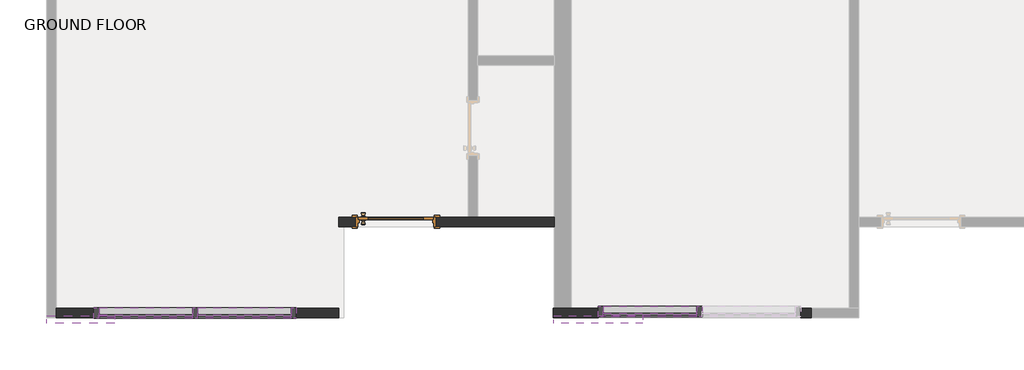
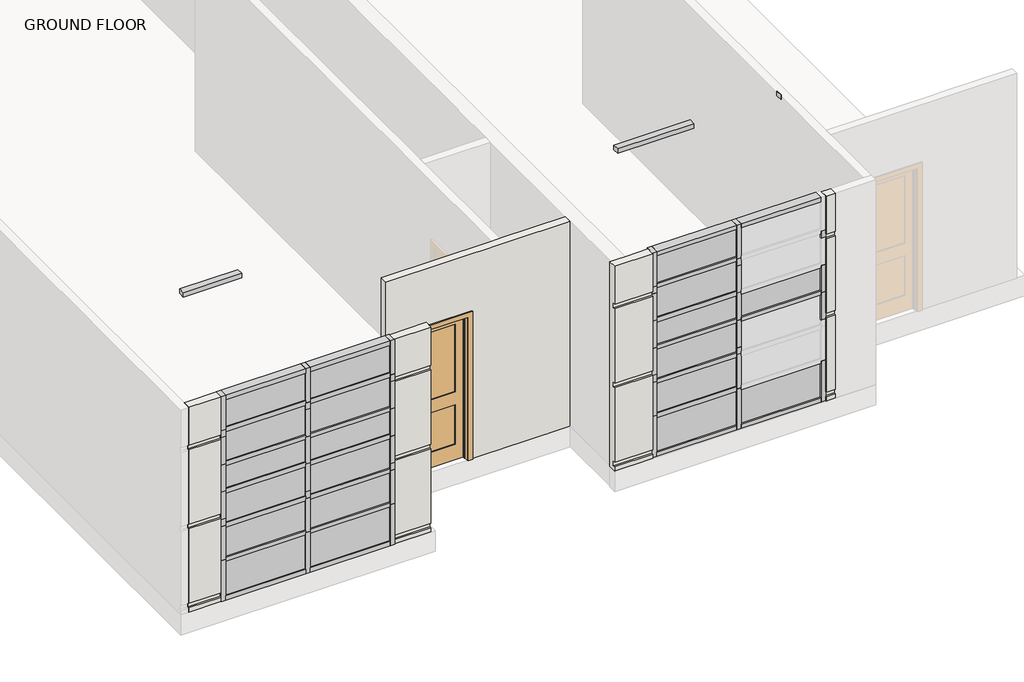
# One storey, part 1 of 4: 68 members, 20 plates, 3 walls, 2 proxies, 1 door.
"""IFC4 building model written with IfcOpenShell, lengths in millimetres."""

from ifc_helpers import new_model, si_unit, frame, origin, place, context, project, spatial, polyline, outline, extrude, faceted_brep, transform, mapped, element, save
from components import door_d4071c8b, member_e6b9f524, member_90c805a2, member_866a01fa, member_7cfea1b5, member_6e77e263, member_47bfaf8a, member_cfc5edb3, member_90750a43, member_7fd687a9, member_fb13da3b, system_panel_glazed_01dbb714, system_panel_glazed_738ee2ab, system_panel_glazed_162183a4, system_panel_glazed_09ecb9ef, system_panel_glazed_28d744da, system_panel_glazed_d671f7fc

model = new_model("IFC4")

# Units and contexts
model_context = context("Model", 3, world=origin())
ifc_project = project(units=[si_unit("LENGTHUNIT", "METRE", prefix="MILLI")], contexts=[model_context])

# Site, building, storey
site = spatial("IfcSite", under=ifc_project)
building = spatial("IfcBuilding", under=site)
storey = spatial("IfcBuildingStorey", under=building, Name="GROUND FLOOR", Elevation=304.8)

# Proxies
placement = place(None, origin())
element("IfcBuildingElementProxy", 1, Name="Reveal 2", ObjectType="Reveal 2", at=placement, inside=storey, context=model_context, shape_type="SweptSolid", body=[
    extrude(outline(polyline([(-18263.2007021, -5496.2840801), (-18263.2007021, -5404.2090801), (-17444.0507021, -5404.2090801), (-17444.0507021, -5496.2840801), (-18263.2007021, -5496.2840801)])), frame((0.0, 0.0, 5072.38), z_axis=(0.0, 0.0, 1.0), x_axis=(1.0, 0.0, 0.0)), (0.0, 0.0, 1.0), 67.7333333),
])
element("IfcBuildingElementProxy", 2, Name="Reveal 2", ObjectType="Reveal 2", at=placement, inside=storey, context=model_context, shape_type="SweptSolid", body=[
    extrude(outline(polyline([(-9849.450702, -5405.2582515), (-9849.450702, -5497.3332515), (-9856.2720515, -5497.3332515), (-9856.2720515, -5405.2582515), (-9849.450702, -5405.2582515)])), frame((0.0, 0.0, 5072.38), z_axis=(0.0, 0.0, 1.0), x_axis=(1.0, 0.0, 0.0)), (0.0, 0.0, 1.0), 67.7333333),
    extrude(outline(polyline([(-11075.4720515, -5405.2582515), (-11075.4720515, -5497.3332515), (-12149.0934009, -5497.3332515), (-12149.0934009, -5405.2582515), (-11075.4720515, -5405.2582515)])), frame((0.0, 0.0, 5072.38), z_axis=(0.0, 0.0, 1.0), x_axis=(1.0, 0.0, 0.0)), (0.0, 0.0, 1.0), 67.7333333),
])

# Door
door_shape = door_d4071c8b(model_context)
element("IfcDoor", 3, ObjectType="Door-Interior-Single-2_Panel-Wood : 36\" x 84\"", at=placement, inside=storey, context=model_context, shape_type="MappedRepresentation", body=[
    mapped(door_shape, transform((-14053.1507021, -4269.409083, 304.8), x_axis=(1.0, 0.0, 0.0), y_axis=(0.0, 1.0, 0.0), z_axis=(0.0, 0.0, 1.0))),
])

# Members
member_shape = member_e6b9f524(model_context)
element("IfcMember", 4, ObjectType="Rectangular Mullion : 2.5\" x 5\" rectangular", at=placement, inside=storey, context=model_context, shape_type="MappedRepresentation", body=[
    mapped(member_shape, transform((-15316.8007021, -5372.4590801, 3352.8), x_axis=(0.0, 0.0, 1.0), y_axis=(0.0, -1.0, 0.0), z_axis=(1.0, 0.0, 0.0))),
])
element("IfcMember", 5, ObjectType="Rectangular Mullion : 2.5\" x 5\" rectangular", at=placement, inside=storey, context=model_context, shape_type="MappedRepresentation", body=[
    mapped(member_shape, transform((-16504.2507021, -5372.4590801, 3352.8), x_axis=(0.0, 0.0, 1.0), y_axis=(0.0, -1.0, 0.0), z_axis=(1.0, 0.0, 0.0))),
])
element("IfcMember", 6, ObjectType="Rectangular Mullion : 2.5\" x 5\" rectangular", at=placement, inside=storey, context=model_context, shape_type="MappedRepresentation", body=[
    mapped(member_shape, transform((-9240.0344894, -5353.4090801, 3352.8), x_axis=(0.0, 0.0, 1.0), y_axis=(0.0, -1.0, 0.0), z_axis=(1.0, 0.0, 0.0))),
])
element("IfcMember", 7, ObjectType="Rectangular Mullion : 2.5\" x 5\" rectangular", at=placement, inside=storey, context=model_context, shape_type="MappedRepresentation", body=[
    mapped(member_shape, transform((-10427.4844894, -5353.4090801, 3352.8), x_axis=(0.0, 0.0, 1.0), y_axis=(0.0, -1.0, 0.0), z_axis=(1.0, 0.0, 0.0))),
])
element("IfcMember", 8, ObjectType="Rectangular Mullion : 2.5\" x 5\" rectangular", at=placement, inside=storey, context=model_context, shape_type="MappedRepresentation", body=[
    mapped(member_shape, transform((-17628.2007021, -5372.4590801, 304.8), x_axis=(0.0, 0.0, -1.0), y_axis=(0.0, -1.0, 0.0), z_axis=(-1.0, 0.0, 0.0))),
])
element("IfcMember", 9, ObjectType="Rectangular Mullion : 2.5\" x 5\" rectangular", at=placement, inside=storey, context=model_context, shape_type="MappedRepresentation", body=[
    mapped(member_shape, transform((-16440.7507021, -5372.4590801, 304.8), x_axis=(0.0, 0.0, -1.0), y_axis=(0.0, -1.0, 0.0), z_axis=(-1.0, 0.0, 0.0))),
])
element("IfcMember", 10, ObjectType="Rectangular Mullion : 2.5\" x 5\" rectangular", at=placement, inside=storey, context=model_context, shape_type="MappedRepresentation", body=[
    mapped(member_shape, transform((-11551.4344894, -5353.4090801, 304.8), x_axis=(0.0, 0.0, -1.0), y_axis=(0.0, -1.0, 0.0), z_axis=(-1.0, 0.0, 0.0))),
])
element("IfcMember", 11, ObjectType="Rectangular Mullion : 2.5\" x 5\" rectangular", at=placement, inside=storey, context=model_context, shape_type="MappedRepresentation", body=[
    mapped(member_shape, transform((-10363.9844894, -5353.4090801, 304.8), x_axis=(0.0, 0.0, -1.0), y_axis=(0.0, -1.0, 0.0), z_axis=(-1.0, 0.0, 0.0))),
])
member_2_shape = member_90c805a2(model_context)
element("IfcMember", 12, ObjectType="Rectangular Mullion : 2.5\" x 5\" rectangular", at=placement, inside=storey, context=model_context, shape_type="MappedRepresentation", body=[
    mapped(member_2_shape, transform((-16472.5007021, -5372.4590801, 1524.0), x_axis=(1.0, 0.0, 0.0), y_axis=(0.0, -1.0, 0.0), z_axis=(0.0, 0.0, -1.0))),
])
element("IfcMember", 13, ObjectType="Rectangular Mullion : 2.5\" x 5\" rectangular", at=placement, inside=storey, context=model_context, shape_type="MappedRepresentation", body=[
    mapped(member_2_shape, transform((-10395.7344894, -5353.4090801, 1524.0), x_axis=(1.0, 0.0, 0.0), y_axis=(0.0, -1.0, 0.0), z_axis=(0.0, 0.0, -1.0))),
])
member_3_shape = member_866a01fa(model_context)
element("IfcMember", 14, ObjectType="Rectangular Mullion : 2.5\" x 5\" rectangular", at=placement, inside=storey, context=model_context, shape_type="MappedRepresentation", body=[
    mapped(member_3_shape, transform((-16504.2507021, -5372.4590801, 1930.4), x_axis=(0.0, 0.0, 1.0), y_axis=(0.0, -1.0, 0.0), z_axis=(1.0, 0.0, 0.0))),
])
element("IfcMember", 15, ObjectType="Rectangular Mullion : 2.5\" x 5\" rectangular", at=placement, inside=storey, context=model_context, shape_type="MappedRepresentation", body=[
    mapped(member_3_shape, transform((-15316.8007021, -5372.4590801, 1930.4), x_axis=(0.0, 0.0, 1.0), y_axis=(0.0, -1.0, 0.0), z_axis=(1.0, 0.0, 0.0))),
])
element("IfcMember", 16, ObjectType="Rectangular Mullion : 2.5\" x 5\" rectangular", at=placement, inside=storey, context=model_context, shape_type="MappedRepresentation", body=[
    mapped(member_3_shape, transform((-16504.2507021, -5372.4590801, 2336.8), x_axis=(0.0, 0.0, 1.0), y_axis=(0.0, -1.0, 0.0), z_axis=(1.0, 0.0, 0.0))),
])
element("IfcMember", 17, ObjectType="Rectangular Mullion : 2.5\" x 5\" rectangular", at=placement, inside=storey, context=model_context, shape_type="MappedRepresentation", body=[
    mapped(member_3_shape, transform((-15316.8007021, -5372.4590801, 2336.8), x_axis=(0.0, 0.0, 1.0), y_axis=(0.0, -1.0, 0.0), z_axis=(1.0, 0.0, 0.0))),
])
element("IfcMember", 18, ObjectType="Rectangular Mullion : 2.5\" x 5\" rectangular", at=placement, inside=storey, context=model_context, shape_type="MappedRepresentation", body=[
    mapped(member_3_shape, transform((-16504.2507021, -5372.4590801, 914.4), x_axis=(0.0, 0.0, 1.0), y_axis=(0.0, -1.0, 0.0), z_axis=(1.0, 0.0, 0.0))),
])
element("IfcMember", 19, ObjectType="Rectangular Mullion : 2.5\" x 5\" rectangular", at=placement, inside=storey, context=model_context, shape_type="MappedRepresentation", body=[
    mapped(member_3_shape, transform((-15316.8007021, -5372.4590801, 914.4), x_axis=(0.0, 0.0, 1.0), y_axis=(0.0, -1.0, 0.0), z_axis=(1.0, 0.0, 0.0))),
])
element("IfcMember", 20, ObjectType="Rectangular Mullion : 2.5\" x 5\" rectangular", at=placement, inside=storey, context=model_context, shape_type="MappedRepresentation", body=[
    mapped(member_3_shape, transform((-16504.2507021, -5372.4590801, 2844.8), x_axis=(0.0, 0.0, 1.0), y_axis=(0.0, -1.0, 0.0), z_axis=(1.0, 0.0, 0.0))),
])
element("IfcMember", 21, ObjectType="Rectangular Mullion : 2.5\" x 5\" rectangular", at=placement, inside=storey, context=model_context, shape_type="MappedRepresentation", body=[
    mapped(member_3_shape, transform((-15316.8007021, -5372.4590801, 2844.8), x_axis=(0.0, 0.0, 1.0), y_axis=(0.0, -1.0, 0.0), z_axis=(1.0, 0.0, 0.0))),
])
element("IfcMember", 22, ObjectType="Rectangular Mullion : 2.5\" x 5\" rectangular", at=placement, inside=storey, context=model_context, shape_type="MappedRepresentation", body=[
    mapped(member_3_shape, transform((-16504.2507021, -5372.4590801, 1422.4), x_axis=(0.0, 0.0, 1.0), y_axis=(0.0, -1.0, 0.0), z_axis=(1.0, 0.0, 0.0))),
])
element("IfcMember", 23, ObjectType="Rectangular Mullion : 2.5\" x 5\" rectangular", at=placement, inside=storey, context=model_context, shape_type="MappedRepresentation", body=[
    mapped(member_3_shape, transform((-15316.8007021, -5372.4590801, 1422.4), x_axis=(0.0, 0.0, 1.0), y_axis=(0.0, -1.0, 0.0), z_axis=(1.0, 0.0, 0.0))),
])
element("IfcMember", 24, ObjectType="Rectangular Mullion : 2.5\" x 5\" rectangular", at=placement, inside=storey, context=model_context, shape_type="MappedRepresentation", body=[
    mapped(member_3_shape, transform((-10427.4844894, -5353.4090801, 1930.4), x_axis=(0.0, 0.0, 1.0), y_axis=(0.0, -1.0, 0.0), z_axis=(1.0, 0.0, 0.0))),
])
element("IfcMember", 25, ObjectType="Rectangular Mullion : 2.5\" x 5\" rectangular", at=placement, inside=storey, context=model_context, shape_type="MappedRepresentation", body=[
    mapped(member_3_shape, transform((-9240.0344894, -5353.4090801, 1930.4), x_axis=(0.0, 0.0, 1.0), y_axis=(0.0, -1.0, 0.0), z_axis=(1.0, 0.0, 0.0))),
])
element("IfcMember", 26, ObjectType="Rectangular Mullion : 2.5\" x 5\" rectangular", at=placement, inside=storey, context=model_context, shape_type="MappedRepresentation", body=[
    mapped(member_3_shape, transform((-10427.4844894, -5353.4090801, 2336.8), x_axis=(0.0, 0.0, 1.0), y_axis=(0.0, -1.0, 0.0), z_axis=(1.0, 0.0, 0.0))),
])
element("IfcMember", 27, ObjectType="Rectangular Mullion : 2.5\" x 5\" rectangular", at=placement, inside=storey, context=model_context, shape_type="MappedRepresentation", body=[
    mapped(member_3_shape, transform((-10427.4844894, -5353.4090801, 914.4), x_axis=(0.0, 0.0, 1.0), y_axis=(0.0, -1.0, 0.0), z_axis=(1.0, 0.0, 0.0))),
])
element("IfcMember", 28, ObjectType="Rectangular Mullion : 2.5\" x 5\" rectangular", at=placement, inside=storey, context=model_context, shape_type="MappedRepresentation", body=[
    mapped(member_3_shape, transform((-10427.4844894, -5353.4090801, 2844.8), x_axis=(0.0, 0.0, 1.0), y_axis=(0.0, -1.0, 0.0), z_axis=(1.0, 0.0, 0.0))),
])
element("IfcMember", 29, ObjectType="Rectangular Mullion : 2.5\" x 5\" rectangular", at=placement, inside=storey, context=model_context, shape_type="MappedRepresentation", body=[
    mapped(member_3_shape, transform((-10427.4844894, -5353.4090801, 1422.4), x_axis=(0.0, 0.0, 1.0), y_axis=(0.0, -1.0, 0.0), z_axis=(1.0, 0.0, 0.0))),
])
member_4_shape = member_7cfea1b5(model_context)
element("IfcMember", 30, ObjectType="Rectangular Mullion : 2.5\" x 5\" rectangular", at=placement, inside=storey, context=model_context, shape_type="MappedRepresentation", body=[
    mapped(member_4_shape, transform((-15253.3007021, -5372.4590801, 1524.0), x_axis=(1.0, 0.0, 0.0), y_axis=(0.0, -1.0, 0.0), z_axis=(0.0, 0.0, -1.0))),
])
element("IfcMember", 31, ObjectType="Rectangular Mullion : 2.5\" x 5\" rectangular", at=placement, inside=storey, context=model_context, shape_type="MappedRepresentation", body=[
    mapped(member_4_shape, transform((-9176.5344894, -5353.4090801, 1524.0), x_axis=(1.0, 0.0, 0.0), y_axis=(0.0, -1.0, 0.0), z_axis=(0.0, 0.0, -1.0))),
])
element("IfcMember", 32, ObjectType="Rectangular Mullion : 2.5\" x 5\" rectangular", at=placement, inside=storey, context=model_context, shape_type="MappedRepresentation", body=[
    mapped(member_4_shape, transform((-17691.7007021, -5372.4590801, 1930.4), x_axis=(-1.0, 0.0, 0.0), y_axis=(0.0, -1.0, 0.0), z_axis=(0.0, 0.0, 1.0))),
])
element("IfcMember", 33, ObjectType="Rectangular Mullion : 2.5\" x 5\" rectangular", at=placement, inside=storey, context=model_context, shape_type="MappedRepresentation", body=[
    mapped(member_4_shape, transform((-11614.9344894, -5353.4090801, 1930.4), x_axis=(-1.0, 0.0, 0.0), y_axis=(0.0, -1.0, 0.0), z_axis=(0.0, 0.0, 1.0))),
])
element("IfcMember", 34, ObjectType="Rectangular Mullion : 2.5\" x 5\" rectangular", at=placement, inside=storey, context=model_context, shape_type="MappedRepresentation", body=[
    mapped(member_2_shape, transform((-16472.5007021, -5372.4590801, 1930.4), x_axis=(1.0, 0.0, 0.0), y_axis=(0.0, -1.0, 0.0), z_axis=(0.0, 0.0, -1.0))),
])
element("IfcMember", 35, ObjectType="Rectangular Mullion : 2.5\" x 5\" rectangular", at=placement, inside=storey, context=model_context, shape_type="MappedRepresentation", body=[
    mapped(member_2_shape, transform((-10395.7344894, -5353.4090801, 1930.4), x_axis=(1.0, 0.0, 0.0), y_axis=(0.0, -1.0, 0.0), z_axis=(0.0, 0.0, -1.0))),
])
element("IfcMember", 36, ObjectType="Rectangular Mullion : 2.5\" x 5\" rectangular", at=placement, inside=storey, context=model_context, shape_type="MappedRepresentation", body=[
    mapped(member_2_shape, transform((-16472.5007021, -5372.4590801, 2336.8), x_axis=(1.0, 0.0, 0.0), y_axis=(0.0, -1.0, 0.0), z_axis=(0.0, 0.0, -1.0))),
])
element("IfcMember", 37, ObjectType="Rectangular Mullion : 2.5\" x 5\" rectangular", at=placement, inside=storey, context=model_context, shape_type="MappedRepresentation", body=[
    mapped(member_2_shape, transform((-10395.7344894, -5353.4090801, 2336.8), x_axis=(1.0, 0.0, 0.0), y_axis=(0.0, -1.0, 0.0), z_axis=(0.0, 0.0, -1.0))),
])
element("IfcMember", 38, ObjectType="Rectangular Mullion : 2.5\" x 5\" rectangular", at=placement, inside=storey, context=model_context, shape_type="MappedRepresentation", body=[
    mapped(member_4_shape, transform((-17691.7007021, -5372.4590801, 2743.2), x_axis=(-1.0, 0.0, 0.0), y_axis=(0.0, -1.0, 0.0), z_axis=(0.0, 0.0, 1.0))),
])
element("IfcMember", 39, ObjectType="Rectangular Mullion : 2.5\" x 5\" rectangular", at=placement, inside=storey, context=model_context, shape_type="MappedRepresentation", body=[
    mapped(member_4_shape, transform((-11614.9344894, -5353.4090801, 2743.2), x_axis=(-1.0, 0.0, 0.0), y_axis=(0.0, -1.0, 0.0), z_axis=(0.0, 0.0, 1.0))),
])
element("IfcMember", 40, ObjectType="Rectangular Mullion : 2.5\" x 5\" rectangular", at=placement, inside=storey, context=model_context, shape_type="MappedRepresentation", body=[
    mapped(member_4_shape, transform((-15253.3007021, -5372.4590801, 1930.4), x_axis=(1.0, 0.0, 0.0), y_axis=(0.0, -1.0, 0.0), z_axis=(0.0, 0.0, -1.0))),
])
element("IfcMember", 41, ObjectType="Rectangular Mullion : 2.5\" x 5\" rectangular", at=placement, inside=storey, context=model_context, shape_type="MappedRepresentation", body=[
    mapped(member_4_shape, transform((-9176.5344894, -5353.4090801, 1930.4), x_axis=(1.0, 0.0, 0.0), y_axis=(0.0, -1.0, 0.0), z_axis=(0.0, 0.0, -1.0))),
])
element("IfcMember", 42, ObjectType="Rectangular Mullion : 2.5\" x 5\" rectangular", at=placement, inside=storey, context=model_context, shape_type="MappedRepresentation", body=[
    mapped(member_4_shape, transform((-15253.3007021, -5372.4590801, 2336.8), x_axis=(1.0, 0.0, 0.0), y_axis=(0.0, -1.0, 0.0), z_axis=(0.0, 0.0, -1.0))),
])
element("IfcMember", 43, ObjectType="Rectangular Mullion : 2.5\" x 5\" rectangular", at=placement, inside=storey, context=model_context, shape_type="MappedRepresentation", body=[
    mapped(member_4_shape, transform((-17691.7007021, -5372.4590801, 2336.8), x_axis=(-1.0, 0.0, 0.0), y_axis=(0.0, -1.0, 0.0), z_axis=(0.0, 0.0, 1.0))),
])
element("IfcMember", 44, ObjectType="Rectangular Mullion : 2.5\" x 5\" rectangular", at=placement, inside=storey, context=model_context, shape_type="MappedRepresentation", body=[
    mapped(member_4_shape, transform((-11614.9344894, -5353.4090801, 2336.8), x_axis=(-1.0, 0.0, 0.0), y_axis=(0.0, -1.0, 0.0), z_axis=(0.0, 0.0, 1.0))),
])
member_5_shape = member_6e77e263(model_context)
element("IfcMember", 45, ObjectType="Rectangular Mullion : 2.5\" x 5\" rectangular", at=placement, inside=storey, context=model_context, shape_type="MappedRepresentation", body=[
    mapped(member_5_shape, transform((-16472.5007021, -5372.4590801, 304.8), x_axis=(1.0, 0.0, 0.0), y_axis=(0.0, -1.0, 0.0), z_axis=(0.0, 0.0, -1.0))),
])
element("IfcMember", 46, ObjectType="Rectangular Mullion : 2.5\" x 5\" rectangular", at=placement, inside=storey, context=model_context, shape_type="MappedRepresentation", body=[
    mapped(member_5_shape, transform((-10395.7344894, -5353.4090801, 304.8), x_axis=(1.0, 0.0, 0.0), y_axis=(0.0, -1.0, 0.0), z_axis=(0.0, 0.0, -1.0))),
])
member_6_shape = member_47bfaf8a(model_context)
element("IfcMember", 47, ObjectType="Rectangular Mullion : 2.5\" x 5\" rectangular", at=placement, inside=storey, context=model_context, shape_type="MappedRepresentation", body=[
    mapped(member_6_shape, transform((-15253.3007021, -5372.4590801, 304.8), x_axis=(1.0, 0.0, 0.0), y_axis=(0.0, -1.0, 0.0), z_axis=(0.0, 0.0, -1.0))),
])
element("IfcMember", 48, ObjectType="Rectangular Mullion : 2.5\" x 5\" rectangular", at=placement, inside=storey, context=model_context, shape_type="MappedRepresentation", body=[
    mapped(member_6_shape, transform((-9176.5344894, -5353.4090801, 304.8), x_axis=(1.0, 0.0, 0.0), y_axis=(0.0, -1.0, 0.0), z_axis=(0.0, 0.0, -1.0))),
])
element("IfcMember", 49, ObjectType="Rectangular Mullion : 2.5\" x 5\" rectangular", at=placement, inside=storey, context=model_context, shape_type="MappedRepresentation", body=[
    mapped(member_6_shape, transform((-17691.7007021, -5372.4590801, 914.4), x_axis=(-1.0, 0.0, 0.0), y_axis=(0.0, -1.0, 0.0), z_axis=(0.0, 0.0, 1.0))),
])
element("IfcMember", 50, ObjectType="Rectangular Mullion : 2.5\" x 5\" rectangular", at=placement, inside=storey, context=model_context, shape_type="MappedRepresentation", body=[
    mapped(member_6_shape, transform((-11614.9344894, -5353.4090801, 914.4), x_axis=(-1.0, 0.0, 0.0), y_axis=(0.0, -1.0, 0.0), z_axis=(0.0, 0.0, 1.0))),
])
member_7_shape = member_cfc5edb3(model_context)
element("IfcMember", 51, ObjectType="Rectangular Mullion : 2.5\" x 5\" rectangular", at=placement, inside=storey, context=model_context, shape_type="MappedRepresentation", body=[
    mapped(member_7_shape, transform((-16472.5007021, -5372.4590801, 2743.2), x_axis=(1.0, 0.0, 0.0), y_axis=(0.0, -1.0, 0.0), z_axis=(0.0, 0.0, -1.0))),
])
element("IfcMember", 52, ObjectType="Rectangular Mullion : 2.5\" x 5\" rectangular", at=placement, inside=storey, context=model_context, shape_type="MappedRepresentation", body=[
    mapped(member_7_shape, transform((-10395.7344894, -5353.4090801, 2743.2), x_axis=(1.0, 0.0, 0.0), y_axis=(0.0, -1.0, 0.0), z_axis=(0.0, 0.0, -1.0))),
])
member_8_shape = member_90750a43(model_context)
element("IfcMember", 53, ObjectType="Rectangular Mullion : 2.5\" x 5\" rectangular", at=placement, inside=storey, context=model_context, shape_type="MappedRepresentation", body=[
    mapped(member_8_shape, transform((-16472.5007021, -5372.4590801, 2844.8), x_axis=(1.0, 0.0, 0.0), y_axis=(0.0, -1.0, 0.0), z_axis=(0.0, 0.0, -1.0))),
])
element("IfcMember", 54, ObjectType="Rectangular Mullion : 2.5\" x 5\" rectangular", at=placement, inside=storey, context=model_context, shape_type="MappedRepresentation", body=[
    mapped(member_8_shape, transform((-10395.7344894, -5353.4090801, 2844.8), x_axis=(1.0, 0.0, 0.0), y_axis=(0.0, -1.0, 0.0), z_axis=(0.0, 0.0, -1.0))),
])
member_9_shape = member_7fd687a9(model_context)
element("IfcMember", 55, ObjectType="Rectangular Mullion : 2.5\" x 5\" rectangular", at=placement, inside=storey, context=model_context, shape_type="MappedRepresentation", body=[
    mapped(member_9_shape, transform((-17691.7007021, -5372.4590801, 3352.8), x_axis=(-1.0, 0.0, 0.0), y_axis=(0.0, -1.0, 0.0), z_axis=(0.0, 0.0, 1.0))),
])
element("IfcMember", 56, ObjectType="Rectangular Mullion : 2.5\" x 5\" rectangular", at=placement, inside=storey, context=model_context, shape_type="MappedRepresentation", body=[
    mapped(member_9_shape, transform((-11614.9344894, -5353.4090801, 3352.8), x_axis=(-1.0, 0.0, 0.0), y_axis=(0.0, -1.0, 0.0), z_axis=(0.0, 0.0, 1.0))),
])
member_10_shape = member_fb13da3b(model_context)
element("IfcMember", 57, ObjectType="Rectangular Mullion : 2.5\" x 5\" rectangular", at=placement, inside=storey, context=model_context, shape_type="MappedRepresentation", body=[
    mapped(member_10_shape, transform((-15253.3007021, -5372.4590801, 2743.2), x_axis=(1.0, 0.0, 0.0), y_axis=(0.0, -1.0, 0.0), z_axis=(0.0, 0.0, -1.0))),
])
element("IfcMember", 58, ObjectType="Rectangular Mullion : 2.5\" x 5\" rectangular", at=placement, inside=storey, context=model_context, shape_type="MappedRepresentation", body=[
    mapped(member_10_shape, transform((-9176.5344894, -5353.4090801, 2743.2), x_axis=(1.0, 0.0, 0.0), y_axis=(0.0, -1.0, 0.0), z_axis=(0.0, 0.0, -1.0))),
])
element("IfcMember", 59, ObjectType="Rectangular Mullion : 2.5\" x 5\" rectangular", at=placement, inside=storey, context=model_context, shape_type="MappedRepresentation", body=[
    mapped(member_9_shape, transform((-15253.3007021, -5372.4590801, 2844.8), x_axis=(1.0, 0.0, 0.0), y_axis=(0.0, -1.0, 0.0), z_axis=(0.0, 0.0, -1.0))),
])
element("IfcMember", 60, ObjectType="Rectangular Mullion : 2.5\" x 5\" rectangular", at=placement, inside=storey, context=model_context, shape_type="MappedRepresentation", body=[
    mapped(member_10_shape, transform((-17691.7007021, -5372.4590801, 2844.8), x_axis=(-1.0, 0.0, 0.0), y_axis=(0.0, -1.0, 0.0), z_axis=(0.0, 0.0, 1.0))),
])
element("IfcMember", 61, ObjectType="Rectangular Mullion : 2.5\" x 5\" rectangular", at=placement, inside=storey, context=model_context, shape_type="MappedRepresentation", body=[
    mapped(member_10_shape, transform((-11614.9344894, -5353.4090801, 2844.8), x_axis=(-1.0, 0.0, 0.0), y_axis=(0.0, -1.0, 0.0), z_axis=(0.0, 0.0, 1.0))),
])
element("IfcMember", 62, ObjectType="Rectangular Mullion : 2.5\" x 5\" rectangular", at=placement, inside=storey, context=model_context, shape_type="MappedRepresentation", body=[
    mapped(member_8_shape, transform((-16472.5007021, -5372.4590801, 914.4), x_axis=(1.0, 0.0, 0.0), y_axis=(0.0, -1.0, 0.0), z_axis=(0.0, 0.0, -1.0))),
])
element("IfcMember", 63, ObjectType="Rectangular Mullion : 2.5\" x 5\" rectangular", at=placement, inside=storey, context=model_context, shape_type="MappedRepresentation", body=[
    mapped(member_8_shape, transform((-10395.7344894, -5353.4090801, 914.4), x_axis=(1.0, 0.0, 0.0), y_axis=(0.0, -1.0, 0.0), z_axis=(0.0, 0.0, -1.0))),
])
element("IfcMember", 64, ObjectType="Rectangular Mullion : 2.5\" x 5\" rectangular", at=placement, inside=storey, context=model_context, shape_type="MappedRepresentation", body=[
    mapped(member_7_shape, transform((-16472.5007021, -5372.4590801, 1422.4), x_axis=(1.0, 0.0, 0.0), y_axis=(0.0, -1.0, 0.0), z_axis=(0.0, 0.0, -1.0))),
])
element("IfcMember", 65, ObjectType="Rectangular Mullion : 2.5\" x 5\" rectangular", at=placement, inside=storey, context=model_context, shape_type="MappedRepresentation", body=[
    mapped(member_7_shape, transform((-10395.7344894, -5353.4090801, 1422.4), x_axis=(1.0, 0.0, 0.0), y_axis=(0.0, -1.0, 0.0), z_axis=(0.0, 0.0, -1.0))),
])
element("IfcMember", 66, ObjectType="Rectangular Mullion : 2.5\" x 5\" rectangular", at=placement, inside=storey, context=model_context, shape_type="MappedRepresentation", body=[
    mapped(member_10_shape, transform((-17691.7007021, -5372.4590801, 1524.0), x_axis=(-1.0, 0.0, 0.0), y_axis=(0.0, -1.0, 0.0), z_axis=(0.0, 0.0, 1.0))),
])
element("IfcMember", 67, ObjectType="Rectangular Mullion : 2.5\" x 5\" rectangular", at=placement, inside=storey, context=model_context, shape_type="MappedRepresentation", body=[
    mapped(member_10_shape, transform((-11614.9344894, -5353.4090801, 1524.0), x_axis=(-1.0, 0.0, 0.0), y_axis=(0.0, -1.0, 0.0), z_axis=(0.0, 0.0, 1.0))),
])
element("IfcMember", 68, ObjectType="Rectangular Mullion : 2.5\" x 5\" rectangular", at=placement, inside=storey, context=model_context, shape_type="MappedRepresentation", body=[
    mapped(member_9_shape, transform((-15253.3007021, -5372.4590801, 914.4), x_axis=(1.0, 0.0, 0.0), y_axis=(0.0, -1.0, 0.0), z_axis=(0.0, 0.0, -1.0))),
])
element("IfcMember", 69, ObjectType="Rectangular Mullion : 2.5\" x 5\" rectangular", at=placement, inside=storey, context=model_context, shape_type="MappedRepresentation", body=[
    mapped(member_10_shape, transform((-15253.3007021, -5372.4590801, 1422.4), x_axis=(1.0, 0.0, 0.0), y_axis=(0.0, -1.0, 0.0), z_axis=(0.0, 0.0, -1.0))),
])
element("IfcMember", 70, ObjectType="Rectangular Mullion : 2.5\" x 5\" rectangular", at=placement, inside=storey, context=model_context, shape_type="MappedRepresentation", body=[
    mapped(member_9_shape, transform((-17691.7007021, -5372.4590801, 1422.4), x_axis=(-1.0, 0.0, 0.0), y_axis=(0.0, -1.0, 0.0), z_axis=(0.0, 0.0, 1.0))),
])
element("IfcMember", 71, ObjectType="Rectangular Mullion : 2.5\" x 5\" rectangular", at=placement, inside=storey, context=model_context, shape_type="MappedRepresentation", body=[
    mapped(member_9_shape, transform((-11614.9344894, -5353.4090801, 1422.4), x_axis=(-1.0, 0.0, 0.0), y_axis=(0.0, -1.0, 0.0), z_axis=(0.0, 0.0, 1.0))),
])

# Plates
system_panel_glazed_shape = system_panel_glazed_01dbb714(model_context)
element("IfcPlate", 72, ObjectType="System Panel : Glazed", at=placement, inside=storey, context=model_context, shape_type="MappedRepresentation", body=[
    mapped(system_panel_glazed_shape, transform((-17066.2257021, -5372.4590801, 1962.15), x_axis=(1.0, 0.0, 0.0), y_axis=(0.0, 1.0, 0.0), z_axis=(0.0, 0.0, 1.0))),
])
element("IfcPlate", 73, ObjectType="System Panel : Glazed", at=placement, inside=storey, context=model_context, shape_type="MappedRepresentation", body=[
    mapped(system_panel_glazed_shape, transform((-15878.7757021, -5372.4590801, 1962.15), x_axis=(1.0, 0.0, 0.0), y_axis=(0.0, 1.0, 0.0), z_axis=(0.0, 0.0, 1.0))),
])
element("IfcPlate", 74, ObjectType="System Panel : Glazed", at=placement, inside=storey, context=model_context, shape_type="MappedRepresentation", body=[
    mapped(system_panel_glazed_shape, transform((-10989.4594894, -5353.4090801, 1962.15), x_axis=(1.0, 0.0, 0.0), y_axis=(0.0, 1.0, 0.0), z_axis=(0.0, 0.0, 1.0))),
])
element("IfcPlate", 75, ObjectType="System Panel : Glazed", at=placement, inside=storey, context=model_context, shape_type="MappedRepresentation", body=[
    mapped(system_panel_glazed_shape, transform((-9802.0094894, -5353.4090801, 1962.15), x_axis=(1.0, 0.0, 0.0), y_axis=(0.0, 1.0, 0.0), z_axis=(0.0, 0.0, 1.0))),
])
system_panel_glazed_2_shape = system_panel_glazed_738ee2ab(model_context)
element("IfcPlate", 76, ObjectType="System Panel : Glazed", at=placement, inside=storey, context=model_context, shape_type="MappedRepresentation", body=[
    mapped(system_panel_glazed_2_shape, transform((-17066.2257021, -5372.4590801, 368.3), x_axis=(1.0, 0.0, 0.0), y_axis=(0.0, 1.0, 0.0), z_axis=(0.0, 0.0, 1.0))),
])
element("IfcPlate", 77, ObjectType="System Panel : Glazed", at=placement, inside=storey, context=model_context, shape_type="MappedRepresentation", body=[
    mapped(system_panel_glazed_2_shape, transform((-15878.7757021, -5372.4590801, 368.3), x_axis=(1.0, 0.0, 0.0), y_axis=(0.0, 1.0, 0.0), z_axis=(0.0, 0.0, 1.0))),
])
element("IfcPlate", 78, ObjectType="System Panel : Glazed", at=placement, inside=storey, context=model_context, shape_type="MappedRepresentation", body=[
    mapped(system_panel_glazed_2_shape, transform((-10989.4594894, -5353.4090801, 368.3), x_axis=(1.0, 0.0, 0.0), y_axis=(0.0, 1.0, 0.0), z_axis=(0.0, 0.0, 1.0))),
])
element("IfcPlate", 79, ObjectType="System Panel : Glazed", at=placement, inside=storey, context=model_context, shape_type="MappedRepresentation", body=[
    mapped(system_panel_glazed_2_shape, transform((-9802.0094894, -5353.4090801, 368.3), x_axis=(1.0, 0.0, 0.0), y_axis=(0.0, 1.0, 0.0), z_axis=(0.0, 0.0, 1.0))),
])
system_panel_glazed_3_shape = system_panel_glazed_162183a4(model_context)
element("IfcPlate", 80, ObjectType="System Panel : Glazed", at=placement, inside=storey, context=model_context, shape_type="MappedRepresentation", body=[
    mapped(system_panel_glazed_3_shape, transform((-17066.2257021, -5372.4590801, 2368.55), x_axis=(1.0, 0.0, 0.0), y_axis=(0.0, 1.0, 0.0), z_axis=(0.0, 0.0, 1.0))),
])
element("IfcPlate", 81, ObjectType="System Panel : Glazed", at=placement, inside=storey, context=model_context, shape_type="MappedRepresentation", body=[
    mapped(system_panel_glazed_3_shape, transform((-15878.7757021, -5372.4590801, 2368.55), x_axis=(1.0, 0.0, 0.0), y_axis=(0.0, 1.0, 0.0), z_axis=(0.0, 0.0, 1.0))),
])
element("IfcPlate", 82, ObjectType="System Panel : Glazed", at=placement, inside=storey, context=model_context, shape_type="MappedRepresentation", body=[
    mapped(system_panel_glazed_3_shape, transform((-10989.4594894, -5353.4090801, 2368.55), x_axis=(1.0, 0.0, 0.0), y_axis=(0.0, 1.0, 0.0), z_axis=(0.0, 0.0, 1.0))),
])
system_panel_glazed_4_shape = system_panel_glazed_09ecb9ef(model_context)
element("IfcPlate", 83, ObjectType="System Panel : Glazed", at=placement, inside=storey, context=model_context, shape_type="MappedRepresentation", body=[
    mapped(system_panel_glazed_4_shape, transform((-17066.2257021, -5372.4590801, 2876.55), x_axis=(1.0, 0.0, 0.0), y_axis=(0.0, 1.0, 0.0), z_axis=(0.0, 0.0, 1.0))),
])
element("IfcPlate", 84, ObjectType="System Panel : Glazed", at=placement, inside=storey, context=model_context, shape_type="MappedRepresentation", body=[
    mapped(system_panel_glazed_4_shape, transform((-15878.7757021, -5372.4590801, 2876.55), x_axis=(1.0, 0.0, 0.0), y_axis=(0.0, 1.0, 0.0), z_axis=(0.0, 0.0, 1.0))),
])
element("IfcPlate", 85, ObjectType="System Panel : Glazed", at=placement, inside=storey, context=model_context, shape_type="MappedRepresentation", body=[
    mapped(system_panel_glazed_4_shape, transform((-10989.4594894, -5353.4090801, 2876.55), x_axis=(1.0, 0.0, 0.0), y_axis=(0.0, 1.0, 0.0), z_axis=(0.0, 0.0, 1.0))),
])
system_panel_glazed_5_shape = system_panel_glazed_28d744da(model_context)
element("IfcPlate", 86, ObjectType="System Panel : Glazed", at=placement, inside=storey, context=model_context, shape_type="MappedRepresentation", body=[
    mapped(system_panel_glazed_5_shape, transform((-17066.2257021, -5372.4590801, 946.15), x_axis=(1.0, 0.0, 0.0), y_axis=(0.0, 1.0, 0.0), z_axis=(0.0, 0.0, 1.0))),
])
element("IfcPlate", 87, ObjectType="System Panel : Glazed", at=placement, inside=storey, context=model_context, shape_type="MappedRepresentation", body=[
    mapped(system_panel_glazed_5_shape, transform((-15878.7757021, -5372.4590801, 946.15), x_axis=(1.0, 0.0, 0.0), y_axis=(0.0, 1.0, 0.0), z_axis=(0.0, 0.0, 1.0))),
])
element("IfcPlate", 88, ObjectType="System Panel : Glazed", at=placement, inside=storey, context=model_context, shape_type="MappedRepresentation", body=[
    mapped(system_panel_glazed_5_shape, transform((-10989.4594894, -5353.4090801, 946.15), x_axis=(1.0, 0.0, 0.0), y_axis=(0.0, 1.0, 0.0), z_axis=(0.0, 0.0, 1.0))),
])
system_panel_glazed_6_shape = system_panel_glazed_d671f7fc(model_context)
element("IfcPlate", 89, ObjectType="System Panel : Glazed", at=placement, inside=storey, context=model_context, shape_type="MappedRepresentation", body=[
    mapped(system_panel_glazed_6_shape, transform((-17066.2257021, -5372.4590801, 1454.15), x_axis=(1.0, 0.0, 0.0), y_axis=(0.0, 1.0, 0.0), z_axis=(0.0, 0.0, 1.0))),
])
element("IfcPlate", 90, ObjectType="System Panel : Glazed", at=placement, inside=storey, context=model_context, shape_type="MappedRepresentation", body=[
    mapped(system_panel_glazed_6_shape, transform((-15878.7757021, -5372.4590801, 1454.15), x_axis=(1.0, 0.0, 0.0), y_axis=(0.0, 1.0, 0.0), z_axis=(0.0, 0.0, 1.0))),
])
element("IfcPlate", 91, ObjectType="System Panel : Glazed", at=placement, inside=storey, context=model_context, shape_type="MappedRepresentation", body=[
    mapped(system_panel_glazed_6_shape, transform((-10989.4594894, -5353.4090801, 1454.15), x_axis=(1.0, 0.0, 0.0), y_axis=(0.0, 1.0, 0.0), z_axis=(0.0, 0.0, 1.0))),
])

# Walls
element("IfcWall", 92, at=placement, inside=storey, context=model_context, shape_type="SweptSolid", body=[
    extrude(outline(polyline([(-5429.6090801, 3352.8), (-5315.3090801, 3352.8), (-5315.3090801, 304.8), (-5429.6090801, 304.8), (-5429.6090801, 368.3), (-5404.2090801, 368.3), (-5404.2090801, 436.0333333), (-5429.6090801, 436.0333333), (-5429.6090801, 1544.32), (-5404.2090801, 1544.32), (-5404.2090801, 1612.0533333), (-5429.6090801, 1612.0533333), (-5429.6090801, 2720.34), (-5404.2090801, 2720.34), (-5404.2090801, 2788.0733333), (-5429.6090801, 2788.0733333), (-5429.6090801, 3352.8)])), frame((-18148.9007021, 0.0, 0.0), z_axis=(1.0, 0.0, 0.0), x_axis=(0.0, 1.0, 0.0)), (0.0, 0.0, 1.0), 457.2),
    extrude(outline(polyline([(-5315.3090801, 3352.8), (-5315.3090801, 304.8), (-5429.6090801, 304.8), (-5429.6090801, 368.3), (-5404.2090801, 368.3), (-5404.2090801, 436.0333333), (-5429.6090801, 436.0333333), (-5429.6090801, 1544.32), (-5404.2090801, 1544.32), (-5404.2090801, 1612.0533333), (-5429.6090801, 1612.0533333), (-5429.6090801, 2720.34), (-5404.2090801, 2720.34), (-5404.2090801, 2788.0733333), (-5429.6090801, 2788.0733333), (-5429.6090801, 3352.8), (-5315.3090801, 3352.8)])), frame((-15253.3007021, 0.0, 0.0), z_axis=(1.0, 0.0, 0.0), x_axis=(0.0, 1.0, 0.0)), (0.0, 0.0, 1.0), 514.35),
])
element("IfcWall", 93, at=placement, inside=storey, context=model_context, shape_type="Brep", body=[
    faceted_brep([(-12154.5007021, -5315.3090801, 304.8), (-12154.5007021, -5315.3090801, 3352.8), (-12143.6860997, -5315.3090801, 3352.8), (-11940.4860997, -5315.3090801, 3352.8), (-11614.9344894, -5315.3090801, 3352.8), (-11614.9344894, -5315.3090801, 304.8), (-11940.4860997, -5315.3090801, 304.8), (-12143.6860997, -5315.3090801, 304.8), (-11614.9344894, -5429.6090801, 3352.8), (-12154.5007021, -5429.6090801, 3352.8), (-12154.5007021, -5429.6090801, 2788.0733333), (-11614.9344894, -5429.6090801, 2788.0733333), (-12154.5007021, -5429.6090801, 304.8), (-11614.9344894, -5429.6090801, 304.8), (-11614.9344894, -5429.6090801, 368.3), (-12154.5007021, -5429.6090801, 368.3), (-12154.5007021, -5429.6090801, 436.0333333), (-11614.9344894, -5429.6090801, 436.0333333), (-11614.9344894, -5429.6090801, 1544.32), (-12154.5007021, -5429.6090801, 1544.32), (-11614.9344894, -5429.6090801, 2720.34), (-12154.5007021, -5429.6090801, 2720.34), (-12154.5007021, -5429.6090801, 1612.0533333), (-11614.9344894, -5429.6090801, 1612.0533333), (-12154.5007021, -5404.2090801, 368.3), (-12154.5007021, -5404.2090801, 436.0333333), (-12154.5007021, -5404.2090801, 1544.32), (-12154.5007021, -5404.2090801, 1612.0533333), (-12154.5007021, -5404.2090801, 2720.34), (-12154.5007021, -5404.2090801, 2788.0733333), (-11614.9344894, -5404.2090801, 2788.0733333), (-11614.9344894, -5404.2090801, 2720.34), (-11614.9344894, -5404.2090801, 1612.0533333), (-11614.9344894, -5404.2090801, 1544.32), (-11614.9344894, -5404.2090801, 436.0333333), (-11614.9344894, -5404.2090801, 368.3)], [[[0, 1, 2, 3, 4, 5, 6, 7]], [[8, 9, 10, 11]], [[12, 13, 14, 15]], [[16, 17, 18, 19]], [[20, 21, 22, 23]], [[12, 0, 7, 6, 5, 13]], [[1, 0, 12, 15, 24, 25, 16, 19, 26, 27, 22, 21, 28, 29, 10, 9]], [[1, 9, 8, 4, 3, 2]], [[5, 4, 8, 11, 30, 31, 20, 23, 32, 33, 18, 17, 34, 35, 14, 13]], [[25, 34, 17, 16]], [[35, 24, 15, 14]], [[34, 25, 24, 35]], [[29, 30, 11, 10]], [[31, 28, 21, 20]], [[30, 29, 28, 31]], [[27, 32, 23, 22]], [[33, 26, 19, 18]], [[32, 27, 26, 33]]]),
    faceted_brep([(-9044.8860997, -5315.3090801, 3352.8), (-9044.8860997, -5315.3090801, 304.8), (-9176.5344894, -5315.3090801, 304.8), (-9176.5344894, -5315.3090801, 3352.8), (-9044.8860997, -5429.6090801, 3352.8), (-9176.5344894, -5429.6090801, 3352.8), (-9176.5344894, -5429.6090801, 2788.0733333), (-9044.8860997, -5429.6090801, 2788.0733333), (-9176.5344894, -5429.6090801, 304.8), (-9044.8860997, -5429.6090801, 304.8), (-9044.8860997, -5429.6090801, 368.3), (-9176.5344894, -5429.6090801, 368.3), (-9176.5344894, -5429.6090801, 436.0333333), (-9044.8860997, -5429.6090801, 436.0333333), (-9044.8860997, -5429.6090801, 1544.32), (-9176.5344894, -5429.6090801, 1544.32), (-9044.8860997, -5429.6090801, 2720.34), (-9176.5344894, -5429.6090801, 2720.34), (-9176.5344894, -5429.6090801, 1612.0533333), (-9044.8860997, -5429.6090801, 1612.0533333), (-9044.8860997, -5404.2090801, 2788.0733333), (-9044.8860997, -5404.2090801, 2720.34), (-9044.8860997, -5404.2090801, 1612.0533333), (-9044.8860997, -5404.2090801, 1544.32), (-9044.8860997, -5404.2090801, 436.0333333), (-9044.8860997, -5404.2090801, 368.3), (-9176.5344894, -5404.2090801, 368.3), (-9176.5344894, -5404.2090801, 436.0333333), (-9176.5344894, -5404.2090801, 1544.32), (-9176.5344894, -5404.2090801, 1612.0533333), (-9176.5344894, -5404.2090801, 2720.34), (-9176.5344894, -5404.2090801, 2788.0733333)], [[[0, 1, 2, 3]], [[4, 5, 6, 7]], [[8, 9, 10, 11]], [[12, 13, 14, 15]], [[16, 17, 18, 19]], [[1, 9, 8, 2]], [[4, 0, 3, 5]], [[1, 0, 4, 7, 20, 21, 16, 19, 22, 23, 14, 13, 24, 25, 10, 9]], [[3, 2, 8, 11, 26, 27, 12, 15, 28, 29, 18, 17, 30, 31, 6, 5]], [[27, 24, 13, 12]], [[25, 26, 11, 10]], [[24, 27, 26, 25]], [[31, 20, 7, 6]], [[21, 30, 17, 16]], [[20, 31, 30, 21]], [[29, 22, 19, 18]], [[23, 28, 15, 14]], [[22, 29, 28, 23]]]),
])
element("IfcWall", 94, at=placement, inside=storey, context=model_context, shape_type="Brep", body=[
    faceted_brep([(-12143.6860997, -4329.734083, 3352.8), (-14738.9507021, -4329.734083, 3352.8), (-14738.9507021, -4329.734083, 304.8), (-14535.7507021, -4329.734083, 304.8), (-14535.7507021, -4329.734083, 2463.8), (-13570.5507021, -4329.734083, 2463.8), (-13570.5507021, -4329.734083, 304.8), (-12143.6860997, -4329.734083, 304.8), (-14738.9507021, -4215.434083, 3352.8), (-13183.2007021, -4215.434083, 3352.8), (-13068.9007021, -4215.434083, 3352.8), (-12143.6860997, -4215.434083, 3352.8), (-12143.6860997, -4215.434083, 304.8), (-13068.9007021, -4215.434083, 304.8), (-13183.2007021, -4215.434083, 304.8), (-13570.5507021, -4215.434083, 304.8), (-13570.5507021, -4215.434083, 2463.8), (-14535.7507021, -4215.434083, 2463.8), (-14535.7507021, -4215.434083, 304.8), (-14738.9507021, -4215.434083, 304.8)], [[[0, 1, 2, 3, 4, 5, 6, 7]], [[8, 9, 10, 11, 12, 13, 14, 15, 16, 17, 18, 19]], [[2, 19, 18, 3]], [[12, 7, 6, 15, 14, 13]], [[1, 0, 11, 10, 9, 8]], [[2, 1, 8, 19]], [[0, 7, 12, 11]], [[5, 16, 15, 6]], [[16, 5, 4, 17]], [[17, 4, 3, 18]]]),
])

save(model, "model.ifc")

# Revit data of these elements
# Type "Door-Interior-Single-2_Panel-Wood : 36\" x 84\""
#   Type Mark = "9"
#   Assembly Code = "C1020300"
#   Analytic Construction = "Wooden"
#   Top Rail = 0' - 4 11/16"
#   Thickness = 0' - 1 3/8"
#   Thermal Resistance (R) = 2.5876 (h·ft²·°F)/BTU
#   Swing Angle [instance default] = 90.00°
#   Stiles = 0' - 4 3/4"
#   Rough Width = 3' - 2"
#   Rough Height = 7' - 1"
#   Lock Rail = 0' - 7 1/2"
#   Height = 7' - 0"
#   Width = 3' - 0"
#   Heat Transfer Coefficient (U) = 0.3865 BTU/(h·ft²·°F)
#   Bottom Rail = 0' - 9 1/8"
#   Trim Material = Cherry
#   Panel Material = Cherry
#   Frame Material = Cherry
#   Door Handle Material = Aluminum
#   Visual Light Transmittance = 0
#   Solar Heat Gain Coefficient = 0
#   Wall Closure = (empty or 0)
#   Function = (empty or 0)
# Type "Rectangular Mullion : 2.5\" x 5\" rectangular"
#   built-in parameter 1007304 = 0.416667 (stored number, unit not read)
#   built-in parameter 1007301 = 0.104167 (stored number, unit not read)
#   built-in parameter 1007300 = 0.104167 (stored number, unit not read)
# Type "System Panel : Glazed"
#   Construction Type Id = "GSP4R"
#   Analytic Construction = "1/8 in Pilkington single glazing"
#   Visual Light Transmittance = 0.9
#   Solar Heat Gain Coefficient = 0.86
#   Heat Transfer Coefficient (U) = 1.18115 BTU/(h·ft²·°F)
#   Define Thermal Properties by = 1
# Type
#   Assembly Code = "B2010"
# Element 3 (IfcDoor, "Door-Interior-Single-2_Panel-Wood : 36\" x 84\"")
#   Swing Angle = 90.00°
#   Phase Created = New Construction
#   Materials on its faces: "Cherry", "Aluminum"
# Elements 4, 5, 6, 7, 8, 9, 10, 11, 12, 13, 14, 15, 16, 17, 18, 19, 20, 21, 22, 23, 24, 25, 26, 27, 28, 29, 30, 31, 32, 33, 34, 35, 36, 37, 38, 39, 40, 41, 42, 43, 44, 45, 46, 47, 48, 49, 50, 51, 52, 53, 54, 55, 56, 57, 58, 59, 60, 61, 62, 63, 64, 65, 66, 67, 68, 69, 70, 71 (IfcMember, "Rectangular Mullion : 2.5\" x 5\" rectangular")
#   Phase Created = New Construction
#   Materials on its faces: "Aluminum"
# Elements 72, 73, 74, 75, 76, 77, 78, 79, 80, 81, 82, 83, 84, 85, 86, 87, 88, 89, 90, 91 (IfcPlate, "System Panel : Glazed")
#   Phase Created = New Construction
#   Materials on its faces: "GARAGE PANEL"
# Element 92 (IfcWall)
#   Top Offset = 0' - 0"
#   Base Offset = 0' - 0"
#   wall height = 10' - 0"
#   Phase Created = New Construction
#   Base Constraint = GROUND FLOOR
#   Top Constraint = FIRST FLOOR
#   Materials on its faces: "Clad - White"
# Element 93 (IfcWall)
#   Top Offset = 0' - 0"
#   Base Offset = 0' - 0"
#   wall height = 10' - 0"
#   Phase Created = New Construction
#   Base Constraint = GROUND FLOOR
#   Top Constraint = FIRST FLOOR
# Element 94 (IfcWall)
#   Top Offset = 0' - 0"
#   Base Offset = 0' - 0"
#   wall height = 10' - 0"
#   Phase Created = New Construction
#   Base Constraint = GROUND FLOOR
#   Top Constraint = FIRST FLOOR
#   Materials on its faces: "red brown cladding"
# Materials
#   "Cherry": class "Wood", colour RGB 226 177 128, transparency 0, Description = "Prunus Serotina", Cost = 0
#   "Aluminum": class "Metal", colour RGB 247 247 247, transparency 0, Description = "Aluminum 6061", Cost = 0
#   "GARAGE PANEL": class "Generic", colour RGB 120 120 120, transparency 0, Cost = 0
#   "Clad - White": class "Wood", colour RGB 242 242 238, transparency 0, Cost = 0
#   "red brown cladding": class "Generic", colour RGB 151 67 57, transparency 0, Cost = 0
